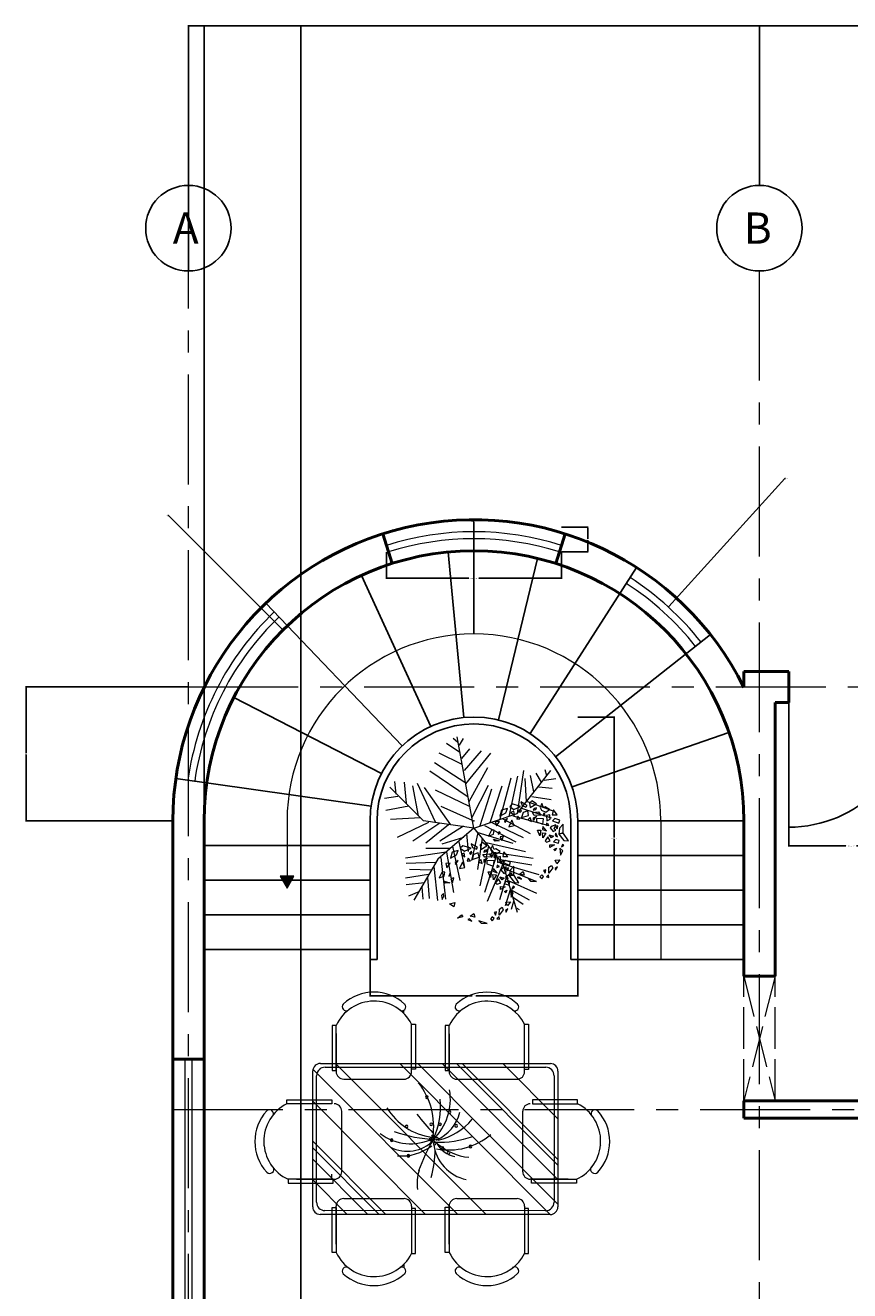
# Model space of a CAD drawing. Units: inches. Extents: x 10696 to 11614, y 5787 to 6498.
# Tile 8 of 9: x 11123 to 11361, y 6132 to 6498. Entities that reach past the tile are written whole.
import ezdxf

# ---------------------------------------------------------------- set-up
doc = ezdxf.new("R2010")
doc.units = ezdxf.units.IN
doc.linetypes.add('ACAD_ISO02W100', pattern=[15, 12, -3])
doc.linetypes.add('CENTER', pattern=[50.8, 31.75, -6.35, 6.35, -6.35])
for name, color, linetype, lineweight in [('A-ANNO-DIMS', 2, 'Continuous', 18), ('A-ANNO-SYMB', 2, 'Continuous', 18), ('A-DOOR', 3, 'Continuous', 25), ('A-FLOR-STRS', 7, 'Continuous', 25), ('A-FURN', 8, 'Continuous', 18), ('A-GLAZ', 4, 'Continuous', 20), ('A-GRID', 1, 'CENTER', 18), ('A-GRID-IDEN', 1, 'Continuous', 25), ('A-WALL', 7, 'Continuous', 50), ('A-WALL-OVHD', 7, 'ACAD_ISO02W100', 18), ('L-PLNT', 94, 'Continuous', 13)]:
    doc.layers.add(name, color=color, linetype=linetype, lineweight=lineweight)
doc.styles.get("Standard").update_dxf_attribs({"font": 'arial.ttf'})
doc.dimstyles.get("Standard").update_dxf_attribs({"dimtxt": 0.18, "dimasz": 0.18, "dimexe": 0.18, "dimexo": 0.0625, "dimgap": 0.09, "dimtad": 0, "dimtih": 1, "dimtoh": 1, "dimdec": 4, "dimzin": 0, "dimdsep": 46, "dimtxsty": 'Standard', "dimcen": 0.09, "dimadec": 0, "dimazin": 0, "dimtfac": 1, "dimtdec": 4, "dimtofl": 0, "dimtmove": 0, "dimatfit": 3, "dimfxl": 1, "dimtolj": 1, "dimtzin": 0, "dimarcsym": 0})

# ---------------------------------------------------------------- blocks, each defined once
blk = doc.blocks.new('*U2')
for p, q in [((-10.186, 53.64), (-13.084, 55.962)), ((0, 0), (-10.5, 57)), ((-9.099, 51.782), (-6.563, 55.962)), ((-8.737, 47.138), (-17.069, 52.711)), ((-7.65, 43.423), (-2.578, 49.46)), ((-5.839, 35.992), (4.667, 48.067)), ((-5.114, 28.097), (-24.676, 40.636)), ((-7.288, 39.707), (-21.778, 46.673)), ((-5.114, 27.632), (10.463, 46.673)), ((-3.665, 19.273), (-27.574, 35.527)), ((-2.941, 16.486), (8.652, 37.85)), ((22.055, 7.198), (27.489, 32.277)), ((27, 9), (48, 36)), ((27.127, 9.056), (31.112, 35.992)), ((35.096, 32.741), (37.27, 22.524)), ((38.719, 34.134), (41.979, 28.561)), ((44.153, 36.456), (45.239, 32.741)), ((-31.5, 4.5), (-52.5, 25.5)), ((-48.585, 21.131), (-49.309, 29.026)), ((-43.513, 28.561), (-42.427, 15.558)), ((-38.442, 26.239), (-34.819, 7.663)), ((-35.544, 28.097), (-24.314, 3.947)), ((-14.533, 2.09), (-30.834, 25.31)), ((-24.314, 23.917), (-2.941, 13.7)), ((-1.129, 6.734), (9.014, 26.704)), ((3.942, 1.625), (11.187, 24.381)), ((10.101, 3.483), (17.708, 26.239)), ((16.259, 5.805), (23.142, 31.348)), ((31.836, 30.883), (32.561, 16.486)), ((40.53, 25.775), (48.862, 24.846)), ((43.791, 29.954), (51.036, 30.883)), ((-47.498, 19.737), (-55.83, 18.344)), ((33.285, 16.486), (48.862, 10.913)), ((36.183, 19.737), (48.137, 17.88)), ((-40.615, 13.7), (-55.105, 10.913)), ((-20.691, 13.7), (-1.129, 4.876)), ((0, 0), (27, 9)), ((29.662, 12.307), (48.137, 6.269)), ((-33.37, 6.269), (-52.207, 5.34)), ((-28.299, 3.483), (-47.86, -5.805)), ((-21.416, 3.018), (-38.079, -8.128)), ((0, 0), (-31.5, 4.5)), ((-15.982, 2.09), (-30.11, -9.521)), ((0, 0), (-22.5, -19.5)), ((-6.563, 1.161), (-21.416, -8.128)), ((0, 0), (18, -22.5)), ((6.478, 1.625), (26.04, -8.592)), ((11.187, 3.483), (30.749, -5.805)), ((18.07, 5.805), (35.096, -3.483)), ((24.229, 7.663), (46.688, 1.625)), ((-6.563, -5.805), (-19.967, -9.985)), ((-4.752, -3.483), (-3.665, -14.629)), ((2.493, -3.019), (-1.491, -20.202)), ((1.769, -2.555), (24.229, -9.521)), ((5.029, -6.27), (2.131, -25.775)), ((-17.431, -15.094), (-42.789, -18.809)), ((-15.257, -12.772), (-30.11, -12.772)), ((-17.069, -15.094), (-12.721, -40.172)), ((-13.446, -11.378), (-8.737, -32.741)), ((-9.461, -8.592), (-6.201, -23.453)), ((9.014, -11.378), (3.58, -35.992)), ((7.565, -9.056), (32.198, -14.629)), ((12.274, -15.094), (36.907, -18.809)), ((-24.314, -21.596), (-42.427, -22.06)), ((-22.5, -19.5), (-37.5, -45)), ((-20.691, -18.345), (-17.793, -44.352)), ((14.085, -16.951), (6.478, -40.172)), ((18.07, -22.524), (8.289, -45.745)), ((16.259, -19.738), (36.183, -22.989)), ((18, -22.5), (27, -52.5)), ((18.433, -22.524), (40.53, -29.026)), ((-28.299, -29.026), (-42.789, -31.348)), ((-26.849, -26.24), (-40.253, -25.775)), ((-29.023, -30.884), (-27.936, -43.887)), ((-25.038, -23.918), (-22.865, -45.281)), ((20.244, -30.419), (15.897, -44.816)), ((19.157, -25.311), (38.719, -33.206)), ((-30.834, -34.135), (-42.427, -35.528)), ((-32.646, -36.921), (-31.921, -44.352)), ((22.78, -37.85), (19.519, -48.532)), ((21.331, -32.741), (39.081, -40.636)), ((22.78, -38.314), (34.372, -44.816)), ((-34.457, -39.708), (-40.978, -42.494)), ((24.591, -45.745), (23.142, -50.854)), ((24.591, -43.423), (30.749, -47.603)), ((26.764, -49.925), (28.213, -50.854))]:
    blk.add_line(p, q)
blk = doc.blocks.new('*U3')
for points in [[(-4.43, 11.05), (-5.18, 10.36), (-3.96, 9.49), (-2.07, 10.36)], [(-2, 11.66), (-1.6, 10.62), (-0.52, 10.1), (-0.18, 10.62), (-0.79, 10.96)], [(1.24, 12), (0.56, 11.31), (0.76, 10.01), (2.52, 11.05)], [(4.14, 11.14), (3.6, 10.01), (4, 9.23), (5.22, 8.71), (6.3, 9.41), (5.08, 10.19), (4.61, 10.01)], [(-5.78, 9.75), (-7.54, 9.23), (-8.01, 7.5), (-6.26, 8.45)], [(-4.84, 8.63), (-3.83, 7.85), (-4.03, 8.97)], [(-2.88, 7.5), (-3.15, 6.64), (-2.27, 6.72)], [(-1.94, 9.49), (-2.48, 8.97), (-2.27, 8.54), (-1.8, 9.06)], [(0.02, 9.06), (-1.33, 8.54), (-1.73, 7.16), (0.29, 7.76)], [(1.37, 8.54), (3.13, 8.8), (3.8, 7.85), (1.91, 7.76)], [(2.59, 9.93), (1.84, 9.75), (1.64, 9.23), (2.32, 9.41)], [(1.71, 6.29), (1.71, 7.07), (2.65, 7.5), (2.11, 6.9)], [(4.61, 8.28), (4.54, 7.76), (4.95, 7.59), (4.95, 8.28)], [(6.43, 7.94), (5.49, 7.68), (5.56, 6.21), (6.5, 6.64)], [(7.45, 9.32), (7.11, 7.94), (8.52, 7.94)], [(-8.14, 6.03), (-9.36, 5.95), (-9.02, 4.73)], [(-5.78, 6.81), (-6.66, 6.21), (-6.52, 5.69)], [(-4.57, 6.38), (-5.45, 4.47), (-3.89, 4.82)], [(0.76, 7.16), (0.09, 6.46), (1.1, 5.95)], [(2.52, 6.81), (2.52, 5.86), (4.41, 5.17), (4.61, 6.72)], [(4.41, 4.56), (4.27, 3.7), (5.49, 3.26)], [(5.49, 5.51), (5.42, 4.82), (6.16, 5.08)], [(8.12, 4.99), (7.11, 4.65), (6.5, 4.13), (7.38, 3.09), (8.12, 3.52), (7.65, 3.87)], [(7.85, 6.81), (7.18, 6.21), (9, 5.51), (9.33, 6.38)], [(8.73, 4.73), (8.19, 4.56), (8.39, 3.87), (8.59, 4.04)], [(10.28, 5.17), (9.2, 4.04), (9, 2.31), (10.48, 0.49), (11.76, 0.41), (10.35, 2.48), (9.33, 2.4), (10.28, 2.83)], [(-11.32, 1.79), (-9.83, 2.31), (-9.63, 3.44), (-10.44, 3.52)], [(-8.21, 0.41), (-9.43, 0.32), (-9.83, 0.84)], [(-8.21, 3.09), (-8.48, 2.31), (-7.87, 2.57)], [(-7, 1.79), (-7.94, 1.53), (-7.47, 0.49)], [(3.53, 1.88), (2.86, 3.52), (3.8, 3.52)], [(4.27, 2.74), (5.29, 2.66), (4.41, 1.27)], [(5.83, 1.53), (5.02, 0.41), (5.49, -0.02), (6.5, 0.41)], [(7.51, 1.71), (6.91, 1.27), (6.23, 2.14)], [(8.12, 0.75), (7.51, 0.15), (8.93, -0.28), (9.13, 0.49)], [(8.19, 2.57), (7.92, 2.05), (8.66, 1.53)], [(-10.03, -2.71), (-10.64, -3.31), (-10.44, -4.44), (-9.9, -3.49)], [(7.78, -0.8), (6.43, -1.5), (6.43, -0.72)], [(8.32, -1.75), (7.98, -2.53), (7.58, -2.1)], [(9.33, -1.75), (9.54, -3.74), (10.14, -2.53)], [(10.08, -0.63), (9.74, -1.32), (10.48, -0.89)], [(-8.28, -5.73), (-6.79, -5.3), (-7, -6.51)], [(6.1, -8.94), (6.16, -7.21), (6.91, -6.69), (7.24, -7.38)], [(8.05, -8.07), (8.59, -7.12), (7.92, -7.55)], [(9.33, -5.13), (8.46, -6.25), (7.98, -5.22)], [(-4.84, -8.85), (-4.43, -9.45), (-5.99, -9.8)], [(-2.54, -10.06), (-3.02, -10.23), (-1.8, -10.67)], [(-2.34, -9.2), (-1.26, -8.5), (-0.99, -9.54)], [(0.22, -10.58), (0.83, -11.27), (2.59, -11.36)], [(4.07, -9.45), (3.53, -9.97), (4.07, -10.58), (4.61, -9.89)], [(5.29, -7.98), (4.61, -8.16), (5.02, -8.94)], [(6.03, -9.45), (5.42, -9.97), (6.16, -10.15)]]:
    blk.add_lwpolyline(points, close=True)
blk = doc.blocks.new('A$C6327331B')
for p, q in [((790.8, 678.3), (790.8, 696.4)), ((790.8, 678.3), (790.8, 696.4)), ((1381.3, 692.8), (1381.3, 686.2)), ((1381.3, 692.8), (1381.3, 686.2)), ((410.1, 615.8), (410, 377)), ((410.1, 615.8), (410, 377)), ((431.6, 615.8), (410.1, 615.8)), ((431.6, 615.8), (410.1, 615.8)), ((431.4, 376.9), (431.6, 615.8)), ((431.4, 376.9), (431.6, 615.8)), ((831.4, 382.9), (831.6, 621.7)), ((831.4, 382.9), (831.6, 621.7)), ((831.6, 621.7), (853, 621.7)), ((831.6, 621.7), (853, 621.7)), ((853, 621.7), (852.9, 382.9)), ((853, 621.7), (852.9, 382.9)), ((1009.3, 615.5), (1009.2, 376.7)), ((1009.3, 615.5), (1009.2, 376.7)), ((1030.7, 615.5), (1009.3, 615.5)), ((1030.7, 615.5), (1009.3, 615.5)), ((1030.6, 376.6), (1030.7, 615.5)), ((1030.6, 376.6), (1030.7, 615.5)), ((1430.6, 382.6), (1430.7, 621.4)), ((1430.6, 382.6), (1430.7, 621.4)), ((1430.7, 621.4), (1452.2, 621.4)), ((1430.7, 621.4), (1452.2, 621.4)), ((1452.2, 621.4), (1452, 382.6)), ((1452.2, 621.4), (1452, 382.6)), ((431.5, 571.8), (431.4, 370.8)), ((431.5, 571.8), (431.4, 370.8)), ((831.4, 370.6), (831.5, 571.6)), ((831.4, 370.6), (831.5, 571.6)), ((1030.7, 571.5), (1030.6, 370.5)), ((1030.7, 571.5), (1030.6, 370.5)), ((1430.6, 370.3), (1430.7, 571.3)), ((1430.6, 370.3), (1430.7, 571.3)), ((347.5, 414), (831.5, 413.8)), ((347.5, 414), (831.5, 413.8)), ((1226.3, -386.4), (428, 414)), ((1226.3, -386.4), (428, 414)), ((1567.1, -386.6), (768.8, 413.8)), ((1567.1, -386.6), (768.8, 413.8)), ((831.5, 413.8), (1567.5, 413.4)), ((1607.1, -331.3), (864.1, 413.8)), ((1607.1, -331.3), (864.1, 413.8)), ((1607.2, -200.8), (994.4, 413.7)), ((1607.2, -200.8), (994.4, 413.7)), ((1009.2, 413.7), (1567.5, 413.4)), ((1607.2, -125.5), (1069.5, 413.7)), ((1607.2, -125.5), (1069.5, 413.7)), ((1607.2, -95.4), (1099.6, 413.6)), ((1607.2, -95.4), (1099.6, 413.6)), ((1607.3, 120.5), (1315.1, 413.5)), ((1607.3, 120.5), (1315.1, 413.5)), ((1415.7, 413.4), (1415.7, 413.5)), ((1415.7, 413.4), (1415.7, 413.5)), ((307.1, -346), (307.5, 374)), ((307.1, -346), (307.5, 374)), ((1075.9, -386.3), (308.5, 383.1)), ((1075.9, -386.3), (308.5, 383.1)), ((327.1, -321), (327.5, 349)), ((372.5, 394), (831.4, 393.8)), ((372.5, 394), (1009.2, 393.7)), ((410, 377), (431.4, 376.9)), ((410, 377), (431.4, 376.9)), ((852.9, 382.9), (831.4, 382.9)), ((852.9, 382.9), (831.4, 382.9)), ((1009.2, 393.7), (1542.5, 393.4)), ((1009.2, 376.7), (1030.6, 376.6)), ((1009.2, 376.7), (1030.6, 376.6)), ((1452, 382.6), (1430.6, 382.6)), ((1452, 382.6), (1430.6, 382.6)), ((1587.5, 348.4), (1587.1, -321.6)), ((1607.5, 373.4), (1607.1, -346.6)), ((1607.5, 373.4), (1607.1, -346.6)), ((471.4, 330.8), (791.4, 330.6)), ((471.4, 330.8), (791.4, 330.6)), ((1070.6, 330.5), (1390.6, 330.3)), ((1070.6, 330.5), (1390.6, 330.3)), ((169.9, 221.5), (408.7, 221.6)), ((169.9, 221.5), (408.7, 221.6)), ((169.9, 200.1), (169.9, 221.5)), ((169.9, 200.1), (169.9, 221.5)), ((905.5, -386.3), (307.4, 213.5)), ((905.5, -386.3), (307.4, 213.5)), ((408.7, 221.6), (408.7, 200.2)), ((408.7, 221.6), (408.7, 200.2)), ((1473.3, 221.6), (1473.3, 200.2)), ((1473.3, 221.6), (1473.3, 200.2)), ((1712.1, 221.5), (1473.3, 221.6)), ((1712.1, 221.5), (1473.3, 221.6)), ((1712.1, 200.1), (1712.1, 221.5)), ((1712.1, 200.1), (1712.1, 221.5)), ((408.7, 200.2), (169.9, 200.1)), ((408.7, 200.2), (169.9, 200.1)), ((461.2, -159.8), (461, 160.2)), ((461.2, -159.8), (461, 160.2)), ((1420.8, -159.8), (1420.9, 160.2)), ((1420.8, -159.8), (1420.9, 160.2)), ((1473.3, 200.2), (1712.1, 200.1)), ((1473.3, 200.2), (1712.1, 200.1)), ((695.1, -386.2), (307.3, 2.7)), ((695.1, -386.2), (307.3, 2.7)), ((44.6, -20.2), (44.5, -20.1)), ((44.6, -20.2), (44.5, -20.1)), ((660, -386.1), (307.3, -32.5)), ((660, -386.1), (307.3, -32.5)), ((1837.4, -20.2), (1837.5, -20.1)), ((1837.4, -20.2), (1837.5, -20.1)), ((599.8, -386.1), (307.2, -92.7)), ((599.8, -386.1), (307.2, -92.7)), ((415.1, -199.8), (176.2, -199.9)), ((415.1, -199.8), (176.2, -199.9)), ((176.2, -199.9), (176.2, -221.3)), ((176.2, -199.9), (176.2, -221.3)), ((220.2, -199.9), (421.2, -199.8)), ((220.2, -199.9), (421.2, -199.8)), ((408.7, -193.6), (408.7, -172.1)), ((408.7, -193.6), (408.7, -172.1)), ((415.1, -221.2), (415.1, -199.8)), ((415.1, -221.2), (415.1, -199.8)), ((1661.8, -199.9), (1460.8, -199.8)), ((1661.8, -199.9), (1460.8, -199.8)), ((1466.9, -221.2), (1466.9, -199.8)), ((1466.9, -221.2), (1466.9, -199.8)), ((1466.9, -199.8), (1705.7, -199.9)), ((1466.9, -199.8), (1705.7, -199.9)), ((1705.7, -199.9), (1705.7, -221.3)), ((1705.7, -199.9), (1705.7, -221.3)), ((176.2, -221.3), (415.1, -221.2)), ((176.2, -221.3), (415.1, -221.2)), ((489.6, -386), (307.2, -203.2)), ((489.6, -386), (307.2, -203.2)), ((1705.7, -221.3), (1466.9, -221.2)), ((1705.7, -221.3), (1466.9, -221.2)), ((471.4, -302.7), (791.4, -302.5)), ((471.4, -302.7), (791.4, -302.5)), ((1070.6, -302.4), (1390.6, -302.2)), ((1070.6, -302.4), (1390.6, -302.2)), ((1567.1, -386.6), (347.1, -386)), ((1567.1, -386.6), (347.1, -386)), ((1542.1, -366.6), (372.1, -366)), ((410.1, -587.7), (410, -348.9)), ((410.1, -587.7), (410, -348.9)), ((410, -348.9), (431.4, -348.9)), ((410, -348.9), (431.4, -348.9)), ((431.5, -543.7), (431.4, -342.7)), ((431.5, -543.7), (431.4, -342.7)), ((431.4, -348.9), (431.6, -587.7)), ((431.4, -348.9), (431.6, -587.7)), ((831.4, -342.5), (831.5, -543.5)), ((831.4, -342.5), (831.5, -543.5)), ((831.4, -354.8), (831.6, -593.6)), ((831.4, -354.8), (831.6, -593.6)), ((852.9, -354.8), (831.4, -354.8)), ((852.9, -354.8), (831.4, -354.8)), ((831.5, -385.7), (864.1, -385.7)), ((831.5, -385.7), (864.1, -385.7)), ((853, -593.6), (852.9, -354.8)), ((853, -593.6), (852.9, -354.8)), ((1009.2, -348.6), (1030.6, -348.5)), ((1009.2, -348.6), (1030.6, -348.5)), ((1009.3, -587.4), (1009.2, -348.6)), ((1009.3, -587.4), (1009.2, -348.6)), ((1030.7, -543.4), (1030.6, -342.4)), ((1030.7, -543.4), (1030.6, -342.4)), ((1030.6, -348.5), (1030.7, -587.4)), ((1030.6, -348.5), (1030.7, -587.4)), ((1415.7, -385.3), (1415.7, -385.4)), ((1415.7, -385.3), (1415.7, -385.4)), ((1430.6, -342.2), (1430.7, -543.2)), ((1430.6, -342.2), (1430.7, -543.2)), ((1430.6, -354.5), (1430.7, -593.3)), ((1430.6, -354.5), (1430.7, -593.3)), ((1452, -354.5), (1430.6, -354.5)), ((1452, -354.5), (1430.6, -354.5)), ((1452.2, -593.3), (1452, -354.5)), ((1452.2, -593.3), (1452, -354.5)), ((431.6, -587.7), (410.1, -587.7)), ((431.6, -587.7), (410.1, -587.7)), ((831.6, -593.6), (853, -593.6)), ((831.6, -593.6), (853, -593.6)), ((1030.7, -587.4), (1009.3, -587.4)), ((1030.7, -587.4), (1009.3, -587.4)), ((1430.7, -593.3), (1452.2, -593.3)), ((1430.7, -593.3), (1452.2, -593.3)), ((790.8, -650.2), (790.8, -668.4)), ((790.8, -650.2), (790.8, -668.4)), ((1381.3, -664.7), (1381.3, -658.1)), ((1381.3, -664.7), (1381.3, -658.1))]:
    blk.add_line(p, q)
for centre, radius, start, end in [((633, 521.6), 222.4, 26.76564, 154.93691), ((633, 521.6), 222.4, 26.76564, 154.93691), ((631.5, 550.5), 241.3, 47.46915, 132.47205), ((631.5, 550.5), 241.3, 47.46915, 132.47205), ((1232.2, 521.3), 222.4, 84.42654, 154.93691), ((1232.2, 521.3), 222.4, 84.42654, 154.93691), ((1230.7, 550.2), 241.3, 47.46915, 132.47205), ((1230.7, 550.2), 241.3, 47.46915, 132.47205), ((1232.2, 521.3), 222.4, 26.76564, 84.42654), ((1232.2, 521.3), 222.4, 26.76564, 84.42654), ((484.3, 714.2), 21.2, 137.64965, 300.34124), ((484.3, 714.2), 21.2, 137.64965, 300.34124), ((779, 714), 21.2, 239.59996, 42.29154), ((779, 714), 21.2, 239.59996, 42.29154), ((1083.4, 713.9), 21.2, 137.64965, 300.34124), ((1083.4, 713.9), 21.2, 137.64965, 300.34124), ((1378.1, 713.7), 21.2, 239.59996, 42.29154), ((1378.1, 713.7), 21.2, 239.59996, 42.29154), ((347.5, 374), 40, 89.9706, 179.9706), ((347.5, 374), 40, 89.9706, 179.9706), ((1567.5, 373.4), 40, 359.9706, 89.9706), ((1567.5, 373.4), 40, 359.9706, 89.9706), ((372.5, 349), 45, 89.9706, 179.9706), ((471.4, 370.8), 40, 179.9706, 269.9706), ((471.4, 370.8), 40, 179.9706, 269.9706), ((791.4, 370.6), 40, 269.9706, 359.9706), ((791.4, 370.6), 40, 269.9706, 359.9706), ((1070.6, 370.5), 40, 179.9706, 269.9706), ((1070.6, 370.5), 40, 179.9706, 269.9706), ((1390.6, 370.3), 40, 269.9706, 359.9706), ((1390.6, 370.3), 40, 269.9706, 359.9706), ((1542.5, 348.4), 45, 359.9706, 89.9706), ((574.1, 79.9), 374.6, 351.24958, 38.23328), ((737.8, 225), 299.2, 314.48606, 9.37622), ((912.6, 235.7), 6.91, 0, 180), ((912.6, 235.7), 6.91, 180, 0), ((586.4, 182.9), 398.1, 335.08876, 5.96372), ((241.3, 0.1), 241.3, 137.52795, 222.53085), ((270.2, 1.6), 222.4, 116.82445, 244.99571), ((270.2, 1.6), 222.4, 116.82445, 244.99571), ((77.6, 147.4), 21.2, 329.65876, 132.35035), ((77.6, 147.4), 21.2, 329.65876, 132.35035), ((421, 160.2), 40, 0.0294, 90.0294), ((421, 160.2), 40, 0.0294, 90.0294), ((983.2, 350.8), 331, 211.31505, 262.13779), ((2460.3, 1443.6), 2062.1, 219.04877, 222.6799), ((873.8, 207.8), 219.3, 294.09558, 346.29534), ((1033, 155.9), 6.91, 0, 180), ((1033, 155.9), 6.91, 180, 0), ((1460.9, 160.2), 40, 89.9706, 179.9706), ((1460.9, 160.2), 40, 89.9706, 179.9706), ((1611.7, 1.6), 222.4, 295.00429, 63.17555), ((1611.7, 1.6), 222.4, 295.00429, 63.17555), ((1804.4, 147.4), 21.2, 47.64965, 210.34124), ((1804.4, 147.4), 21.2, 47.64965, 210.34124), ((1640.7, 0.1), 241.3, 317.46915, 42.47205), ((1640.7, 0.1), 241.3, 317.46915, 42.47205), ((805, 79.9), 6.91, 0, 180), ((805, 79.9), 6.91, 180, 0), ((934.8, 91.3), 6.91, 0, 180), ((934.8, 91.3), 6.91, 180, 0), ((897.1, 334.6), 335.6, 283.04524, 319.77663), ((982.3, 91.3), 6.91, 0, 180), ((982.3, 91.3), 6.91, 180, 0), ((1067.8, 83.7), 6.91, 0, 180), ((1067.8, 83.7), 6.91, 180, 0), ((826.9, 258.5), 270.1, 233.32313, 295.76326), ((725.8, 7.7), 6.91, 0, 180), ((725.8, 7.7), 6.91, 180, 0), ((807.8, 143), 194.5, 242.99086, 315.91017), ((985.1, 750.7), 739.8, 250.5249, 267.82437), ((1747.6, -469.5), 933.6, 148.98728, 160.36101), ((931.7, 11.5), 6.91, 0, 180), ((931.7, 11.5), 6.91, 180, 0), ((944.3, 26.7), 6.91, 0, 180), ((944.3, 26.7), 6.91, 180, 0), ((947.5, 3.9), 6.91, 0, 180), ((947.5, 3.9), 6.91, 180, 0), ((970.7, 574.8), 578.8, 268.32856, 288.729), ((966.5, 15.3), 6.91, 0, 180), ((966.5, 15.3), 6.91, 180, 0), ((1030.3, 292.7), 337.4, 258.55155, 310.98153), ((776.7, 191.6), 268.2, 265.87406, 306.95584), ((392.7, -33), 564.4, 343.85612, 359.11051), ((953.8, -11.3), 6.91, 0, 180), ((953.8, -11.3), 6.91, 180, 0), ((1167.7, 15.7), 221.9, 186.99045, 258.02836), ((1090.6, 62.7), 145.4, 208.89012, 258.45792), ((1166.2, 212.9), 298.2, 228.7581, 263.8624), ((995, -34.1), 6.91, 0, 180), ((995, -34.1), 6.91, 180, 0), ((1026.7, -60.7), 6.91, 0, 180), ((1026.7, -60.7), 6.91, 180, 0), ((1143.8, -26.5), 6.91, 0, 180), ((1143.8, -26.5), 6.91, 180, 0), ((814.5, -75.9), 6.91, 0, 180), ((814.5, -75.9), 6.91, 180, 0), ((79, -146.7), 22.5, 226.37763, 29.88821), ((79, -146.7), 22.5, 226.37763, 29.88821), ((421.2, -159.8), 40, 270.0294, 0.0294), ((421.2, -159.8), 40, 270.0294, 0.0294), ((1112.9, -226), 252.6, 162.94564, 186.48138), ((1460.8, -159.8), 40, 179.9706, 269.9706), ((1460.8, -159.8), 40, 179.9706, 269.9706), ((1803, -146.7), 22.5, 150.11179, 313.62237), ((1803, -146.7), 22.5, 150.11179, 313.62237), ((372.1, -321), 45, 179.9706, 269.9706), ((471.4, -342.7), 40, 90.0294, 180.0294), ((471.4, -342.7), 40, 90.0294, 180.0294), ((791.4, -342.5), 40, 0.0294, 90.0294), ((791.4, -342.5), 40, 0.0294, 90.0294), ((1070.6, -342.4), 40, 90.0294, 180.0294), ((1070.6, -342.4), 40, 90.0294, 180.0294), ((1390.6, -342.2), 40, 0.0294, 90.0294), ((1390.6, -342.2), 40, 0.0294, 90.0294), ((1542.1, -321.6), 45, 269.9706, 359.9706), ((347.1, -346), 40, 179.9706, 269.9706), ((347.1, -346), 40, 179.9706, 269.9706), ((1567.1, -346.6), 40, 269.9706, 359.9706), ((1567.1, -346.6), 40, 269.9706, 359.9706), ((633, -493.5), 222.4, 205.06309, 333.23436), ((633, -493.5), 222.4, 205.06309, 333.23436), ((1232.2, -493.2), 222.4, 205.06309, 275.57346), ((1232.2, -493.2), 222.4, 205.06309, 275.57346), ((1232.2, -493.2), 222.4, 275.57346, 333.23436), ((1232.2, -493.2), 222.4, 275.57346, 333.23436), ((484.3, -686.1), 21.2, 59.65876, 222.35035), ((484.3, -686.1), 21.2, 59.65876, 222.35035), ((779, -686), 21.2, 317.70846, 120.40004), ((779, -686), 21.2, 317.70846, 120.40004), ((1083.4, -685.8), 21.2, 59.65876, 222.35035), ((1083.4, -685.8), 21.2, 59.65876, 222.35035), ((1378.1, -685.6), 21.2, 317.70846, 120.40004), ((1378.1, -685.6), 21.2, 317.70846, 120.40004), ((631.5, -522.4), 241.3, 227.52795, 312.53085), ((631.5, -522.4), 241.3, 227.52795, 312.53085), ((1230.7, -522.1), 241.3, 227.52795, 312.53085), ((1230.7, -522.1), 241.3, 227.52795, 312.53085)]:
    blk.add_arc(centre, radius, start, end)
at = {"width": 0.8, "flags": 9}
for tag in ['XSIZE', 'YSIZE']:
    blk.add_attdef(tag, (945.2, 11.4), '', height=0.23, rotation=180, dxfattribs=at)
blk = doc.blocks.new('DOOR-SINGLE-36-KITCHEN')
blk.add_line((0, 36), (0, 0))
blk.add_arc((0, 36), 36, 270, 0)
blk = doc.blocks.new('WIN-GLAZ-72')
for p, q in [((0, 72), (0, 0)), ((2, 72), (2, 0))]:
    blk.add_line(p, q)
blk = doc.blocks.new('WIN-ARC-CROWN')
for radius in [83.5, 81.5]:
    blk.add_arc((25.29, -77.67), radius, 72.3705, 107.6295)
blk = doc.blocks.new('WIN-ARC-WEST')
for radius in [83.5, 81.5]:
    blk.add_arc((82.66, -11.5), radius, 133.6902, 171.8873)
blk = doc.blocks.new('WIN-ARC-EAST')
for radius in [83.5, 81.5]:
    blk.add_arc((-44.03, -50.4), radius, 38.1972, 57.2958)
blk = doc.blocks.new('OPENING-OVHD-36X9')
for p, q in [((0, 0), (0, 36)), ((9, 36), (0, 0)), ((0, 36), (9, 0)), ((9, 0), (9, 36))]:
    blk.add_line(p, q)
blk = doc.blocks.new('STAIR-HANDRAIL-RETURN')
for p, q in [((0, 0), (0, 40)), ((60, 0), (60, 40)), ((2, 0), (0, 0)), ((58, 0), (60, 0))]:
    blk.add_line(p, q)
blk.add_lwpolyline([(2, 0), (2, 40, -1), (58, 40), (58, 0)], format="xyb")
blk.add_arc((30, 40), 30, 0, 180)
blk = doc.blocks.new('*D48')
at = {"layer": 'A-ANNO-DIMS', "color": 0, "lineweight": -2, "transparency": 16777216}
for p, q in [((11343.77, 6266.01), (11343.77, 6260.49)), ((11379.77, 6266.01), (11379.77, 6260.49)), ((11343.95, 6260.67), (11360.24, 6260.67)), ((11379.59, 6260.67), (11363.29, 6260.67))]:
    blk.add_line(p, q, dxfattribs=at)
at = {"layer": 'A-ANNO-DIMS', "color": 0, "transparency": 16777216}
for points in [[(11343.95, 6260.7), (11343.95, 6260.64), (11343.77, 6260.67)], [(11379.59, 6260.7), (11379.59, 6260.64), (11379.77, 6260.67)]]:
    blk.add_solid(points, dxfattribs=at)
at = {"layer": 'Defpoints', "color": 0, "transparency": 16777216}
for p in [(11343.77, 6266.07), (11379.77, 6266.07), (11379.77, 6260.67)]:
    blk.add_point(p, dxfattribs=at)
at = {"layer": 'A-ANNO-DIMS', "color": 0, "transparency": 16777216, "insert": (11361.77, 6260.67), "char_height": 0.18, "attachment_point": 5}
blk.add_mtext('\\A1;KITCHEN DOOR 36 TYP.', dxfattribs=at)
blk = doc.blocks.new('*D52')
at = {"layer": 'A-ANNO-DIMS', "color": 0, "lineweight": -2, "transparency": 16777216}
for p, q in [((11227.48, 6345.48), (11227.48, 6337.77)), ((11278.06, 6345.48), (11278.06, 6337.77)), ((11227.66, 6337.95), (11251.31, 6337.95)), ((11277.88, 6337.95), (11254.22, 6337.95))]:
    blk.add_line(p, q, dxfattribs=at)
at = {"layer": 'A-ANNO-DIMS', "color": 0, "transparency": 16777216}
for points in [[(11227.66, 6337.98), (11227.66, 6337.92), (11227.48, 6337.95)], [(11277.88, 6337.98), (11277.88, 6337.92), (11278.06, 6337.95)]]:
    blk.add_solid(points, dxfattribs=at)
at = {"layer": 'Defpoints', "color": 0, "transparency": 16777216}
for p in [(11227.48, 6345.54), (11278.06, 6345.54), (11278.06, 6337.95)]:
    blk.add_point(p, dxfattribs=at)
at = {"layer": 'A-ANNO-DIMS', "color": 0, "transparency": 16777216, "insert": (11252.77, 6337.95), "char_height": 0.18, "attachment_point": 5}
blk.add_mtext('\\A1;CROWN LIGHT 51 TYP.', dxfattribs=at)
blk = doc.blocks.new('*D53')
at = {"layer": 'A-ANNO-DIMS', "color": 0, "lineweight": -2, "transparency": 16777216}
for p, q in [((11278.12, 6352.68), (11285.82, 6352.68)), ((11285.64, 6352.5), (11285.64, 6349.29)), ((11285.64, 6345.72), (11285.64, 6348.93)), ((11278.12, 6345.54), (11285.82, 6345.54))]:
    blk.add_line(p, q, dxfattribs=at)
at = {"layer": 'A-ANNO-DIMS', "color": 0, "transparency": 16777216}
for points in [[(11285.61, 6352.5), (11285.67, 6352.5), (11285.64, 6352.68)], [(11285.61, 6345.72), (11285.67, 6345.72), (11285.64, 6345.54)]]:
    blk.add_solid(points, dxfattribs=at)
at = {"layer": 'Defpoints', "color": 0, "transparency": 16777216}
for p in [(11278.06, 6352.68), (11285.64, 6352.68), (11278.06, 6345.54)]:
    blk.add_point(p, dxfattribs=at)
at = {"layer": 'A-ANNO-DIMS', "color": 0, "transparency": 16777216, "insert": (11285.64, 6349.11), "char_height": 0.18, "attachment_point": 5}
blk.add_mtext('\\A1;7 TYP.', dxfattribs=at)
blk = doc.blocks.new('*D68')
at = {"layer": 'A-ANNO-DIMS', "color": 0, "lineweight": -2, "transparency": 16777216}
for p, q in [((11282.83, 6297.87), (11293.45, 6297.87)), ((11293.27, 6297.69), (11293.27, 6263.05)), ((11293.27, 6228.05), (11293.27, 6262.69)), ((11282.83, 6227.87), (11293.45, 6227.87))]:
    blk.add_line(p, q, dxfattribs=at)
at = {"layer": 'A-ANNO-DIMS', "color": 0, "transparency": 16777216}
for points in [[(11293.24, 6297.69), (11293.3, 6297.69), (11293.27, 6297.87)], [(11293.24, 6228.05), (11293.3, 6228.05), (11293.27, 6227.87)]]:
    blk.add_solid(points, dxfattribs=at)
at = {"layer": 'Defpoints', "color": 0, "transparency": 16777216}
for p in [(11282.77, 6297.87), (11293.27, 6297.87), (11282.77, 6227.87)]:
    blk.add_point(p, dxfattribs=at)
at = {"layer": 'A-ANNO-DIMS', "color": 0, "transparency": 16777216, "insert": (11293.27, 6262.87), "char_height": 0.18, "attachment_point": 5}
blk.add_mtext('\\A1;HANDRAIL 70 TYP.', dxfattribs=at)
blk = doc.blocks.new('*D69')
at = {"layer": 'A-ANNO-DIMS', "color": 0, "lineweight": -2, "transparency": 16777216}
for p, q in [((11222.77, 6227.81), (11222.77, 6217.19)), ((11282.77, 6227.81), (11282.77, 6217.19)), ((11222.95, 6217.37), (11252.24, 6217.37)), ((11282.59, 6217.37), (11253.3, 6217.37))]:
    blk.add_line(p, q, dxfattribs=at)
at = {"layer": 'A-ANNO-DIMS', "color": 0, "transparency": 16777216}
for points in [[(11222.95, 6217.4), (11222.95, 6217.34), (11222.77, 6217.37)], [(11282.59, 6217.4), (11282.59, 6217.34), (11282.77, 6217.37)]]:
    blk.add_solid(points, dxfattribs=at)
at = {"layer": 'Defpoints', "color": 0, "transparency": 16777216}
for p in [(11222.77, 6227.87), (11282.77, 6227.87), (11282.77, 6217.37)]:
    blk.add_point(p, dxfattribs=at)
at = {"layer": 'A-ANNO-DIMS', "color": 0, "transparency": 16777216, "insert": (11252.77, 6217.37), "char_height": 0.18, "attachment_point": 5}
blk.add_mtext('\\A1;60 TYP.', dxfattribs=at)
blk = doc.blocks.new('*D73')
at = {"layer": 'A-ANNO-DIMS', "color": 0, "lineweight": -2, "transparency": 16777216}
for p, q in [((11170.2, 6306.57), (11123.18, 6306.57)), ((11123.36, 6306.39), (11123.36, 6287.4)), ((11123.36, 6268.05), (11123.36, 6287.04)), ((11165.7, 6267.87), (11123.18, 6267.87))]:
    blk.add_line(p, q, dxfattribs=at)
at = {"layer": 'A-ANNO-DIMS', "color": 0, "transparency": 16777216}
for points in [[(11123.33, 6306.39), (11123.39, 6306.39), (11123.36, 6306.57)], [(11123.33, 6268.05), (11123.39, 6268.05), (11123.36, 6267.87)]]:
    blk.add_solid(points, dxfattribs=at)
at = {"layer": 'Defpoints', "color": 0, "transparency": 16777216}
for p in [(11123.36, 6306.57), (11170.27, 6306.57), (11165.77, 6267.87)]:
    blk.add_point(p, dxfattribs=at)
at = {"layer": 'A-ANNO-DIMS', "color": 0, "transparency": 16777216, "insert": (11123.36, 6287.22), "char_height": 0.18, "attachment_point": 5}
blk.add_mtext('\\A1;38.7', dxfattribs=at)
blk = doc.blocks.new('*D77')
at = {"layer": 'A-ANNO-DIMS', "color": 0, "lineweight": -2, "transparency": 16777216}
for p, q in [((11170.27, 6451.45), (11170.27, 6497.62)), ((11170.45, 6497.44), (11252.49, 6497.44)), ((11335.09, 6497.44), (11253.05, 6497.44)), ((11335.27, 6451.45), (11335.27, 6497.62))]:
    blk.add_line(p, q, dxfattribs=at)
at = {"layer": 'A-ANNO-DIMS', "color": 0, "transparency": 16777216}
for points in [[(11170.45, 6497.47), (11170.45, 6497.41), (11170.27, 6497.44)], [(11335.09, 6497.47), (11335.09, 6497.41), (11335.27, 6497.44)]]:
    blk.add_solid(points, dxfattribs=at)
at = {"layer": 'Defpoints', "color": 0, "transparency": 16777216}
for p in [(11335.27, 6497.44), (11170.27, 6451.39), (11335.27, 6451.39)]:
    blk.add_point(p, dxfattribs=at)
at = {"layer": 'A-ANNO-DIMS', "color": 0, "transparency": 16777216, "insert": (11252.77, 6497.44), "char_height": 0.18, "attachment_point": 5}
blk.add_mtext('\\A1;165', dxfattribs=at)
blk = doc.blocks.new('*D78')
at = {"layer": 'A-ANNO-DIMS', "color": 0, "lineweight": -2, "transparency": 16777216}
for p, q in [((11335.27, 6451.45), (11335.27, 6497.62)), ((11335.45, 6497.44), (11360.19, 6497.44)), ((11385.59, 6497.44), (11360.84, 6497.44)), ((11385.77, 6451.45), (11385.77, 6497.62))]:
    blk.add_line(p, q, dxfattribs=at)
at = {"layer": 'A-ANNO-DIMS', "color": 0, "transparency": 16777216}
for points in [[(11335.45, 6497.47), (11335.45, 6497.41), (11335.27, 6497.44)], [(11385.59, 6497.47), (11385.59, 6497.41), (11385.77, 6497.44)]]:
    blk.add_solid(points, dxfattribs=at)
at = {"layer": 'Defpoints', "color": 0, "transparency": 16777216}
for p in [(11385.77, 6497.44), (11335.27, 6451.39), (11385.77, 6451.39)]:
    blk.add_point(p, dxfattribs=at)
at = {"layer": 'A-ANNO-DIMS', "color": 0, "transparency": 16777216, "insert": (11360.52, 6497.44), "char_height": 0.18, "attachment_point": 5}
blk.add_mtext('\\A1;50.5', dxfattribs=at)
blk = doc.blocks.new('*D80')
at = {"layer": 'A-ANNO-DIMS', "color": 0, "lineweight": -2, "transparency": 16777216}
for p, q in [((11170.27, 6426.74), (11170.27, 6497.62)), ((11170.45, 6497.44), (11328.98, 6497.44)), ((11488.09, 6497.44), (11329.56, 6497.44)), ((11488.27, 6426.74), (11488.27, 6497.62))]:
    blk.add_line(p, q, dxfattribs=at)
at = {"layer": 'A-ANNO-DIMS', "color": 0, "transparency": 16777216}
for points in [[(11170.45, 6497.47), (11170.45, 6497.41), (11170.27, 6497.44)], [(11488.09, 6497.47), (11488.09, 6497.41), (11488.27, 6497.44)]]:
    blk.add_solid(points, dxfattribs=at)
at = {"layer": 'Defpoints', "color": 0, "transparency": 16777216}
for p in [(11488.27, 6497.44), (11170.27, 6426.68), (11488.27, 6426.68)]:
    blk.add_point(p, dxfattribs=at)
at = {"layer": 'A-ANNO-DIMS', "color": 0, "transparency": 16777216, "insert": (11329.27, 6497.44), "char_height": 0.18, "attachment_point": 5}
blk.add_mtext('\\A1;318', dxfattribs=at)
blk = doc.blocks.new('*D95')
at = {"layer": 'A-ANNO-DIMS', "color": 0, "lineweight": -2, "transparency": 16777216}
for p, q in [((11174.77, 5961.13), (11174.77, 6497.62)), ((11174.95, 6497.44), (11188.55, 6497.44)), ((11202.59, 6497.44), (11188.99, 6497.44)), ((11202.77, 5961.13), (11202.77, 6497.62))]:
    blk.add_line(p, q, dxfattribs=at)
at = {"layer": 'A-ANNO-DIMS', "color": 0, "transparency": 16777216}
for points in [[(11174.95, 6497.47), (11174.95, 6497.41), (11174.77, 6497.44)], [(11202.59, 6497.47), (11202.59, 6497.41), (11202.77, 6497.44)]]:
    blk.add_solid(points, dxfattribs=at)
at = {"layer": 'Defpoints', "color": 0, "transparency": 16777216}
for p in [(11202.77, 6497.44), (11174.77, 5961.07), (11202.77, 5961.07)]:
    blk.add_point(p, dxfattribs=at)
at = {"layer": 'A-ANNO-DIMS', "color": 0, "transparency": 16777216, "insert": (11188.77, 6497.44), "char_height": 0.18, "attachment_point": 5}
blk.add_mtext('\\A1;28', dxfattribs=at)
blk = doc.blocks.new('*D102')
at = {"layer": 'A-ANNO-DIMS', "color": 0, "lineweight": -2, "transparency": 16777216}
for p, q in [((11164.34, 6356.12), (11164.52, 6356.12)), ((11164.52, 6356.12), (11197.49, 6323.15)), ((11252.68, 6267.87), (11252.86, 6267.87)), ((11252.77, 6267.78), (11252.77, 6267.96))]:
    blk.add_line(p, q, dxfattribs=at)
at = {"layer": 'A-ANNO-DIMS', "color": 0, "transparency": 16777216}
blk.add_solid([(11197.51, 6323.17), (11197.46, 6323.13), (11197.61, 6323.02)], dxfattribs=at)
at = {"layer": 'Defpoints', "color": 0, "transparency": 16777216}
for p in [(11197.61, 6323.02), (11252.77, 6267.87)]:
    blk.add_point(p, dxfattribs=at)
at = {"layer": 'A-ANNO-DIMS', "color": 0, "transparency": 16777216, "insert": (11164.04, 6356.12), "char_height": 0.18, "attachment_point": 5}
blk.add_mtext('\\A1;R78', dxfattribs=at)
blk = doc.blocks.new('*D103')
at = {"layer": 'A-ANNO-DIMS', "color": 0, "lineweight": -2, "transparency": 16777216}
for p, q in [((11252.59, 6354.27), (11252.77, 6354.27)), ((11252.77, 6354.27), (11252.77, 6322.05)), ((11252.68, 6267.87), (11252.86, 6267.87)), ((11252.77, 6267.78), (11252.77, 6267.96))]:
    blk.add_line(p, q, dxfattribs=at)
at = {"layer": 'A-ANNO-DIMS', "color": 0, "transparency": 16777216}
blk.add_solid([(11252.8, 6322.05), (11252.74, 6322.05), (11252.77, 6321.87)], dxfattribs=at)
at = {"layer": 'Defpoints', "color": 0, "transparency": 16777216}
for p in [(11252.77, 6321.87), (11252.77, 6267.87)]:
    blk.add_point(p, dxfattribs=at)
at = {"layer": 'A-ANNO-DIMS', "color": 0, "transparency": 16777216, "insert": (11252.28, 6354.27), "char_height": 0.18, "attachment_point": 5}
blk.add_mtext('\\A1;R54', dxfattribs=at)
blk = doc.blocks.new('*D105')
at = {"layer": 'A-ANNO-DIMS', "color": 0, "lineweight": -2, "transparency": 16777216}
for p, q in [((11342.6, 6366.76), (11309.04, 6329.81)), ((11342.78, 6366.76), (11342.6, 6366.76)), ((11252.68, 6267.87), (11252.86, 6267.87)), ((11252.77, 6267.78), (11252.77, 6267.96))]:
    blk.add_line(p, q, dxfattribs=at)
at = {"layer": 'A-ANNO-DIMS', "color": 0, "transparency": 16777216}
blk.add_solid([(11309.01, 6329.83), (11309.06, 6329.79), (11308.91, 6329.67)], dxfattribs=at)
at = {"layer": 'Defpoints', "color": 0, "transparency": 16777216}
for p in [(11308.91, 6329.67), (11252.77, 6267.87)]:
    blk.add_point(p, dxfattribs=at)
at = {"layer": 'A-ANNO-DIMS', "color": 0, "transparency": 16777216, "insert": (11343.39, 6366.76), "char_height": 0.18, "attachment_point": 5}
blk.add_mtext('\\A1;3X R83.5', dxfattribs=at)

msp = doc.modelspace()

# ---------------------------------------------------------------- hatches: boundary and pattern name
at = {"layer": 'A-ANNO-SYMB'}
h = msp.add_hatch(color=256, dxfattribs=at)
h.dxf.hatch_style = 1
h.paths.add_polyline_path([(11200.758, 6251.921), (11196.776, 6251.921), (11198.767, 6248.473)])

# ---------------------------------------------------------------- linework, layer by layer
for p, q in [((11198.767, 6267.869), (11198.767, 6267.869)), ((11198.767, 6267.869), (11198.767, 6251.921)), ((11306.767, 6267.869), (11306.767, 6227.869))]:
    msp.add_line(p, q, dxfattribs=at)
msp.add_lwpolyline([(11198.767, 6248.473), (11200.758, 6251.921), (11196.776, 6251.921)], close=True, dxfattribs=at)
msp.add_arc((11252.767, 6267.869), 54, 0, 180, dxfattribs=at)
at = {"layer": 'A-FLOR-STRS'}
for p, q in [((11249.896, 6297.731), (11245.301, 6345.51)), ((11259.825, 6297.027), (11271.116, 6343.68)), ((11268.977, 6293.113), (11299.774, 6341.077)), ((11240.283, 6295.147), (11220.308, 6338.794)), ((11232.045, 6289.561), (11192.671, 6330.777)), ((11276.344, 6286.42), (11321.14, 6321.667)), ((11226.088, 6281.587), (11183.4, 6303.536)), ((11281.116, 6277.684), (11326.474, 6293.39)), ((11223.068, 6272.102), (11166.638, 6280.146)), ((11282.767, 6267.869), (11330.767, 6267.869)), ((11222.767, 6260.772), (11174.767, 6260.772)), ((11282.767, 6257.869), (11330.767, 6257.869)), ((11197.44, 6250.772), (11174.767, 6250.772)), ((11222.767, 6250.772), (11200.095, 6250.772)), ((11282.767, 6247.869), (11330.767, 6247.869)), ((11222.767, 6240.772), (11174.767, 6240.772)), ((11282.767, 6237.869), (11330.767, 6237.869)), ((11222.767, 6230.772), (11174.767, 6230.772)), ((11282.767, 6227.869), (11330.767, 6227.869))]:
    msp.add_line(p, q, dxfattribs=at)
at = {"layer": 'A-GRID'}
for p, q in [((11170.267, 5857.07), (11170.267, 6426.679)), ((11335.267, 5887.07), (11335.267, 6426.679)), ((11170.267, 6306.57), (11554.26, 6306.57)), ((11165.767, 6184.57), (11554.26, 6184.57))]:
    msp.add_line(p, q, dxfattribs=at)
at = {"layer": 'A-GRID-IDEN'}
for centre in [(11170.267, 6439.033), (11335.267, 6439.033)]:
    msp.add_circle(centre, 12.353, dxfattribs=at)
at = {"layer": 'A-WALL'}
for p, q in [((11229.144, 6342.205), (11226.419, 6350.783)), ((11276.391, 6342.205), (11279.116, 6350.783)), ((11330.767, 6311.07), (11343.767, 6311.07)), ((11330.767, 6306.404), (11330.767, 6311.07)), ((11343.767, 6302.07), (11343.767, 6311.07)), ((11339.767, 6302.07), (11343.767, 6302.07)), ((11339.767, 6223.07), (11339.767, 6302.07)), ((11165.767, 5857.07), (11165.767, 6267.869)), ((11174.767, 5961.07), (11174.767, 6267.869)), ((11330.767, 6223.07), (11330.767, 6267.869)), ((11330.767, 6223.07), (11339.767, 6223.07)), ((11174.767, 6199.055), (11165.767, 6199.055)), ((11330.767, 6187.07), (11387.767, 6187.07)), ((11330.767, 6182.07), (11330.767, 6187.07)), ((11330.767, 6182.07), (11383.767, 6182.07))]:
    msp.add_line(p, q, dxfattribs=at)
for radius, start in [(87, 26.29156), (78, 0)]:
    msp.add_arc((11252.767, 6267.869), radius, start, 180, dxfattribs=at)

# ---------------------------------------------------------------- block references
at = {"layer": 'A-DOOR'}
msp.add_blockref('DOOR-SINGLE-36-KITCHEN', (11343.767, 6266.07), dxfattribs=at)
at = {"layer": 'A-FLOR-STRS'}
msp.add_blockref('STAIR-HANDRAIL-RETURN', (11222.767, 6227.869), dxfattribs=at)
at = {"layer": 'A-FURN', "xscale": 0.0544898626987332, "yscale": 0.0544898626987332, "zscale": 0.0544898626987332}
msp.add_blockref('A$C6327331B', (11189.451, 6175.292), dxfattribs=at)
at = {"layer": 'A-GLAZ'}
for name, p in [('WIN-ARC-CROWN', (11227.479, 6345.541)), ('WIN-ARC-EAST', (11296.802, 6318.266)), ('WIN-ARC-WEST', (11170.103, 6279.37)), ('WIN-GLAZ-72', (11169.267, 6127.055))]:
    msp.add_blockref(name, p, dxfattribs=at)
at = {"layer": 'A-WALL-OVHD'}
msp.add_blockref('OPENING-OVHD-36X9', (11330.767, 6187.07), dxfattribs=at)
at = {"layer": 'L-PLNT', "xscale": 0.4627879235944911, "yscale": 0.4627879235944911, "zscale": 0.4627879235944911}
msp.add_blockref('*U2', (11252.779, 6265.824), dxfattribs=at)
at = {"layer": 'L-PLNT'}
for p in [(11268.291, 6261.726), (11254.002, 6249.621)]:
    msp.add_blockref('*U3', p, dxfattribs=at)

# ---------------------------------------------------------------- texts
at = {"layer": 'A-GRID-IDEN', "char_height": 9, "attachment_point": 1}
for s, insert in [('A', (11165.757, 6443.573)), ('B', (11330.757, 6443.573))]:
    msp.add_mtext_dynamic_manual_height_columns(s, width=18.12678, gutter_width=12.5, heights=[0], dxfattribs=dict(at, insert=insert))

# ---------------------------------------------------------------- dimensions: what is measured, and where the dimension line sits
at = {"layer": 'A-ANNO-DIMS'}
for base, p1, p2, override, picture, middle in [((11335.267, 6497.443), (11170.267, 6451.386), (11335.267, 6451.386), {"dimdec": 0, "dimlfac": 1, "dimrnd": 0, "dimzin": 0, "dimdsep": 46, "dimlunit": 2}, '*D77', (11252.767, 6497.443)), ((11488.267, 6497.443), (11170.267, 6426.679), (11488.267, 6426.679), {"dimdec": 0, "dimlfac": 1, "dimrnd": 0, "dimzin": 0, "dimdsep": 46, "dimlunit": 2}, '*D80', (11329.267, 6497.443)), ((11202.767, 6497.443), (11174.767, 5961.07), (11202.767, 5961.07), {"dimdec": 0, "dimlfac": 1, "dimrnd": 0, "dimzin": 0, "dimdsep": 46, "dimlunit": 2}, '*D95', (11188.767, 6497.443)), ((11385.767, 6497.443), (11335.267, 6451.386), (11385.767, 6451.386), {"dimdec": 1, "dimlfac": 1, "dimrnd": 0, "dimzin": 0, "dimdsep": 46, "dimlunit": 2}, '*D78', (11360.517, 6497.443))]:
    dim = msp.add_linear_dim(base=base, p1=p1, p2=p2, dimstyle='Standard', override=override, dxfattribs=at)
    dim.commit()
    dim.dimension.update_dxf_attribs({"geometry": picture, "text_midpoint": middle})
dim = msp.add_radius_dim(center=(11252.767, 6267.869), mpoint=(11308.914, 6329.673), text='3X <>', dimstyle='Standard', override={"dimdec": 1, "dimlfac": 1, "dimrnd": 0, "dimzin": 0, "dimdsep": 46, "dimlunit": 2}, dxfattribs=at)
dim.commit()
dim.dimension.update_dxf_attribs({"geometry": '*D105', "text_midpoint": (11343.386, 6366.756), "dimtype": 164})
for mpoint, picture, middle in [((11197.613, 6323.023), '*D102', (11164.035, 6356.115)), ((11252.767, 6321.869), '*D103', (11252.282, 6354.269))]:
    dim = msp.add_radius_dim(center=(11252.767, 6267.869), mpoint=mpoint, dimstyle='Standard', override={"dimdec": 0, "dimlfac": 1, "dimrnd": 0, "dimzin": 0, "dimdsep": 46, "dimlunit": 2}, dxfattribs=at)
    dim.commit()
    dim.dimension.update_dxf_attribs({"geometry": picture, "text_midpoint": middle, "dimtype": 164})
for base, p1, p2, text, picture, middle in [((11285.643, 6352.676), (11278.056, 6345.541), (11278.056, 6352.676), '<> TYP.', '*D53', (11285.643, 6349.108)), ((11293.267, 6297.869), (11282.767, 6227.869), (11282.767, 6297.869), 'HANDRAIL <> TYP.', '*D68', (11293.267, 6262.869))]:
    dim = msp.add_linear_dim(base=base, p1=p1, p2=p2, angle=90, text=text, dimstyle='Standard', override={"dimdec": 0, "dimlfac": 1, "dimrnd": 0, "dimzin": 0, "dimdsep": 46, "dimlunit": 2}, dxfattribs=at)
    dim.commit()
    dim.dimension.update_dxf_attribs({"geometry": picture, "text_midpoint": middle})
for base, p1, p2, text, picture, middle in [((11278.056, 6337.954), (11227.479, 6345.541), (11278.056, 6345.541), 'CROWN LIGHT <> TYP.', '*D52', (11252.767, 6337.954)), ((11379.767, 6260.67), (11343.767, 6266.07), (11379.767, 6266.07), 'KITCHEN DOOR <> TYP.', '*D48', (11361.767, 6260.67)), ((11282.767, 6217.369), (11222.767, 6227.869), (11282.767, 6227.869), '<> TYP.', '*D69', (11252.767, 6217.369))]:
    dim = msp.add_linear_dim(base=base, p1=p1, p2=p2, text=text, dimstyle='Standard', override={"dimdec": 0, "dimlfac": 1, "dimrnd": 0, "dimzin": 0, "dimdsep": 46, "dimlunit": 2}, dxfattribs=at)
    dim.commit()
    dim.dimension.update_dxf_attribs({"geometry": picture, "text_midpoint": middle})
dim = msp.add_linear_dim(base=(11123.364, 6306.57), p1=(11165.767, 6267.869), p2=(11170.267, 6306.57), angle=90, dimstyle='Standard', override={"dimdec": 1, "dimlfac": 1, "dimrnd": 0, "dimzin": 0, "dimdsep": 46, "dimlunit": 2}, dxfattribs=at)
dim.commit()
dim.dimension.update_dxf_attribs({"geometry": '*D73', "text_midpoint": (11123.364, 6287.219)})

doc.saveas('drawing.dxf')
